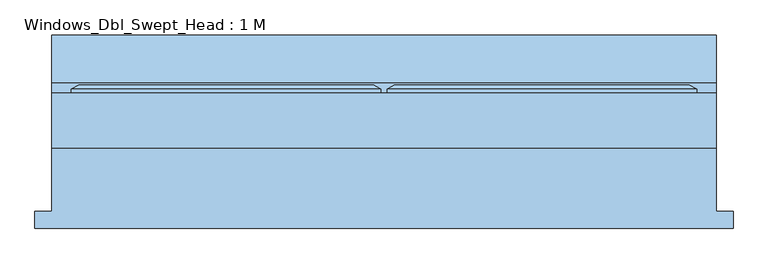
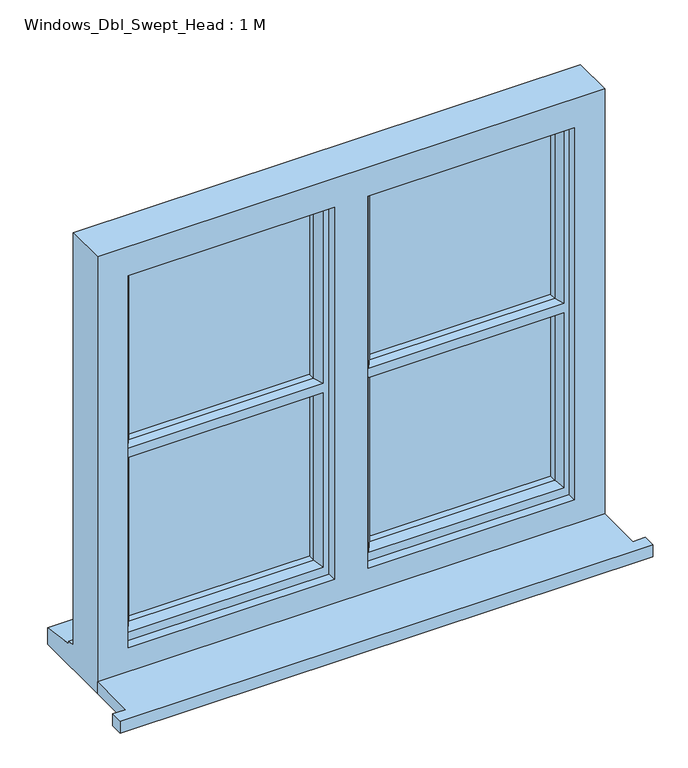
"""IFC4 building model written with IfcOpenShell, lengths in millimetres: window geometry, Windows_Dbl_Swept_Head : 1 M."""

from ifc_helpers import new_model, si_unit, frame, origin, place, context, project, spatial, polyline, circle_curve, outline, extrude, faceted_brep, source, transform, mapped, element, save
from ifc_brep_helpers import plane_surface, revolved_surface, advanced_brep


def windows_dbl_swept_head_1_m_37dff1ae(model_context):
    return source(origin(), model_context, "Body", "SolidModel", [
        extrude(outline(polyline([(-810.0, -130.8434322), (-810.0, -105.8434322), (-785.0, -105.8434322), (-785.0, -10.2434322), (215.0, -10.2434322), (215.0, -105.8434322), (240.0, -105.8434322), (240.0, -130.8434322), (-810.0, -130.8434322)])), frame((0.0, 0.0, 1200.0), z_axis=(0.0, 0.0, 1.0), x_axis=(1.0, 0.0, 0.0)), (0.0, 0.0, 1.0), 25.0),
        extrude(outline(polyline([(145.1480377, 36.7565678), (-240.0, 36.7565678), (-240.0, 60.7565678), (145.1480377, 60.7565678), (145.1480377, 36.7565678)])), frame((0.0, 0.0, 1293.0), z_axis=(0.0, 0.0, 1.0), x_axis=(1.0, 0.0, 0.0)), (0.0, 0.0, 1.0), 365.5),
        extrude(outline(polyline([(145.1480377, 36.7565678), (-240.0, 36.7565678), (-240.0, 60.7565678), (145.1480377, 60.7565678), (145.1480377, 36.7565678)])), frame((0.0, 0.0, 1674.5), z_axis=(0.0, 0.0, 1.0), x_axis=(1.0, 0.0, 0.0)), (0.0, 0.0, 1.0), 365.5),
        extrude(outline(polyline([(-330.0, 36.7565678), (-715.0, 36.7565678), (-715.0, 60.7565678), (-330.0, 60.7565678), (-330.0, 36.7565678)])), frame((0.0, 0.0, 1674.5), z_axis=(0.0, 0.0, 1.0), x_axis=(1.0, 0.0, 0.0)), (0.0, 0.0, 1.0), 365.5),
        extrude(outline(polyline([(-330.0, 36.7565678), (-715.1480377, 36.7565678), (-715.1480377, 60.7565678), (-330.0, 60.7565678), (-330.0, 36.7565678)])), frame((0.0, 0.0, 1292.8519623), z_axis=(0.0, 0.0, 1.0), x_axis=(1.0, 0.0, 0.0)), (0.0, 0.0, 1.0), 365.6480377),
        faceted_brep([(-785.0, -10.2434322, 1200.0), (215.0, -10.2434322, 1200.0), (215.0, -10.2434322, 2110.0), (-785.0, -10.2434322, 2110.0), (-318.0, -10.2434322, 2050.0), (-318.0, -10.2434322, 1275.0), (-725.0, -10.2434322, 1275.0), (-725.0, -10.2434322, 2050.0), (-252.0, -10.2434322, 2050.0), (155.0, -10.2434322, 2050.0), (155.0, -10.2434322, 1275.0), (-252.0, -10.2434322, 1275.0), (-785.0, 72.7565678, 2110.0), (-785.0, 72.7565678, 1251.0), (-785.0, 87.7565678, 1249.68767), (-785.0, 87.7565678, 1244.7449676), (-785.0, 160.2565678, 1233.8088847), (-785.0, 160.2565678, 1200.0), (215.0, 72.7565678, 2110.0), (215.0, 72.7565678, 1251.0), (-745.0, 72.7565678, 2070.0), (-745.0, 72.7565678, 1263.0), (-300.0, 72.7565678, 1263.0), (-300.0, 72.7565678, 2070.0), (-270.0, 72.7565678, 2070.0), (-270.0, 72.7565678, 1263.0), (175.0, 72.7565678, 1263.0), (175.0, 72.7565678, 2070.0), (-745.0, 7.7565678, 2070.0), (-745.0, 7.7565678, 1263.0), (-300.0, 7.7565678, 2070.0), (-300.0, 7.7565678, 1263.0), (-318.0, 7.7565678, 2050.0), (-725.0, 7.7565678, 2050.0), (-725.0, 7.7565678, 1275.0), (-318.0, 7.7565678, 1275.0), (-270.0, 7.7565678, 2070.0), (175.0, 7.7565678, 2070.0), (175.0, 7.7565678, 1263.0), (-270.0, 7.7565678, 1263.0), (155.0, 7.7565678, 2050.0), (-252.0, 7.7565678, 2050.0), (-252.0, 7.7565678, 1275.0), (155.0, 7.7565678, 1275.0), (215.0, 160.2565678, 1200.0), (215.0, 160.2565678, 1233.8088847), (215.0, 87.7565678, 1244.7449676), (215.0, 87.7565678, 1249.68767)], [[[0, 1, 2, 3], [4, 5, 6, 7], [8, 9, 10, 11]], [[0, 3, 12, 13, 14, 15, 16, 17]], [[13, 12, 18, 19], [20, 21, 22, 23], [24, 25, 26, 27]], [[21, 20, 28, 29]], [[28, 30, 31, 29], [32, 33, 34, 35]], [[36, 37, 38, 39], [40, 41, 42, 43]], [[33, 7, 6, 34]], [[12, 3, 2, 18]], [[28, 20, 23, 30]], [[27, 37, 36, 24]], [[7, 33, 32, 4]], [[40, 9, 8, 41]], [[19, 18, 2, 1, 44, 45, 46, 47]], [[27, 26, 38, 37]], [[9, 40, 43, 10]], [[23, 22, 31, 30]], [[25, 24, 36, 39]], [[41, 8, 11, 42]], [[4, 32, 35, 5]], [[44, 1, 0, 17]], [[45, 44, 17, 16]], [[46, 45, 16, 15]], [[47, 46, 15, 14]], [[19, 47, 14, 13]], [[22, 21, 29, 31]], [[26, 25, 39, 38]], [[11, 10, 43, 42]], [[35, 34, 6, 5]]]),
        advanced_brep(
        [(-280.0, 72.7565678, 2080.0), (-280.0, 78.5300705, 2080.0), (-280.0, 78.5300705, 1253.0), (-280.0, 72.7565678, 1253.0), (-270.0, 7.7565678, 2070.0), (-270.0, 72.7565678, 2070.0), (-270.0, 72.7565678, 1263.0), (-270.0, 7.7565678, 1263.0), (-230.0, 22.2494677, 2030.0), (-240.1480377, 7.7565678, 2040.1480377), (-240.1480377, 7.7565678, 1676.3519623), (-230.0, 22.2494677, 1681.5), (-240.1480377, 7.7565678, 1292.8519623), (-230.0, 22.2494677, 1303.0), (-230.0, 22.2494677, 1651.5), (-240.1480377, 7.7565678, 1656.6480377), (-230.0, 36.7565678, 2030.0), (-230.0, 36.7565678, 1681.5), (-230.0, 36.7565678, 1303.0), (-230.0, 36.7565678, 1651.5), (-240.0, 60.7565678, 2040.0), (-240.0, 36.7565678, 2040.0), (-240.0, 36.7565678, 1674.5), (-240.0, 60.7565678, 1674.5), (-240.0, 36.7565678, 1293.0), (-240.0, 60.7565678, 1293.0), (-240.0, 60.7565678, 1658.5), (-240.0, 36.7565678, 1658.5), (-230.0, 60.7565678, 1303.0), (-230.0, 78.5300705, 1303.0), (-230.0, 78.5300705, 1651.5), (-230.0, 60.7565678, 1651.5), (-230.0, 60.7565678, 1681.5), (-230.0, 78.5300705, 1681.5), (-230.0, 78.5300705, 2000.791203), (-230.0, 60.7565678, 2000.791203), (-247.4457548, 84.3035732, 2047.4457548), (-230.0, 78.5300705, 2030.0), (-235.0, 80.1847718, 1681.5), (-247.4457548, 84.3035732, 1669.0542452), (-247.4457548, 84.3035732, 1285.5542452), (-247.4457548, 84.3035732, 1663.9457548), (-235.0, 80.1847718, 1651.5), (-269.2153903, 84.3035732, 2069.2153903), (-269.2153903, 84.3035732, 1263.7846097), (185.0, 78.5300705, 1253.0), (185.0, 72.7565678, 1253.0), (175.0, 72.7565678, 1263.0), (175.0, 7.7565678, 1263.0), (145.1480377, 7.7565678, 1292.8519623), (135.0, 22.2494677, 1303.0), (135.0, 36.7565678, 1303.0), (145.0, 36.7565678, 1293.0), (145.0, 60.7565678, 1293.0), (135.0, 60.7565678, 1303.0), (135.0, 78.5300705, 1303.0), (152.4457548, 84.3035732, 1285.5542452), (174.2153903, 84.3035732, 1263.7846097), (185.0, 78.5300705, 2080.0), (185.0, 72.7565678, 2080.0), (175.0, 72.7565678, 2070.0), (175.0, 7.7565678, 2070.0), (145.1480377, 7.7565678, 1656.6480377), (135.0, 22.2494677, 1651.5), (145.1480377, 7.7565678, 2040.1480377), (135.0, 22.2494677, 2030.0), (135.0, 22.2494677, 1681.5), (145.1480377, 7.7565678, 1676.3519623), (135.0, 36.7565678, 1651.5), (135.0, 36.7565678, 2030.0), (135.0, 36.7565678, 1681.5), (145.0, 36.7565678, 1658.5), (145.0, 60.7565678, 1658.5), (145.0, 36.7565678, 2040.0), (145.0, 60.7565678, 2040.0), (145.0, 60.7565678, 1674.5), (145.0, 36.7565678, 1674.5), (135.0, 60.7565678, 1651.5), (135.0, 78.5300705, 1651.5), (135.0, 78.5300705, 1681.5), (135.0, 60.7565678, 1681.5), (135.0, 60.7565678, 2000.791203), (135.0, 78.5300705, 2000.791203), (140.0, 80.1847718, 1651.5), (152.4457548, 84.3035732, 1663.9457548), (135.0, 78.5300705, 2030.0), (152.4457548, 84.3035732, 2047.4457548), (152.4457548, 84.3035732, 1669.0542452), (140.0, 80.1847718, 1681.5), (174.2153903, 84.3035732, 2069.2153903)],
        [
            (0, 1),
            (1, 2),
            (2, 3),
            (3, 0),
            (4, 5),
            (5, 6),
            (6, 7),
            (7, 4),
            (8, 9),
            (9, 10),
            (10, 11),
            (11, 8),
            (12, 13),
            (13, 14),
            (14, 15),
            (15, 12),
            (16, 8),
            (11, 17),
            (17, 16),
            (13, 18),
            (18, 19),
            (19, 14),
            (20, 21),
            (21, 22),
            (22, 23),
            (23, 20),
            (24, 25),
            (25, 26),
            (26, 27),
            (27, 24),
            (28, 29),
            (29, 30),
            (30, 31),
            (31, 28),
            (32, 33),
            (33, 34),
            (34, 35),
            (35, 32),
            (36, 37),
            (37, 34),
            (33, 38),
            (38, 39),
            (39, 36),
            (29, 40),
            (40, 41),
            (41, 42),
            (42, 30),
            (1, 43),
            (43, 44),
            (44, 2),
            (2, 45),
            (45, 46),
            (46, 3),
            (6, 47),
            (47, 48),
            (48, 7),
            (12, 49),
            (49, 50),
            (50, 13),
            (50, 51),
            (51, 18),
            (24, 52),
            (52, 53),
            (53, 25),
            (28, 54),
            (54, 55),
            (55, 29),
            (55, 56),
            (56, 40),
            (44, 57),
            (57, 45),
            (45, 58),
            (58, 59),
            (59, 46),
            (47, 60),
            (60, 61),
            (61, 48),
            (49, 62),
            (62, 63),
            (63, 50),
            (64, 65),
            (65, 66),
            (66, 67),
            (67, 64),
            (63, 68),
            (68, 51),
            (65, 69),
            (69, 70),
            (70, 66),
            (52, 71),
            (71, 72),
            (72, 53),
            (73, 74),
            (74, 75),
            (75, 76),
            (76, 73),
            (54, 77),
            (77, 78),
            (78, 55),
            (79, 80),
            (80, 81),
            (81, 82),
            (82, 79),
            (78, 83),
            (83, 84),
            (84, 56),
            (85, 86),
            (86, 87),
            (87, 88),
            (88, 79),
            (82, 85),
            (57, 89),
            (89, 58),
            (0, 59),
            (58, 1),
            (5, 60),
            (4, 61),
            (15, 62),
            (9, 64),
            (67, 10),
            (8, 65),
            (16, 69),
            (27, 71),
            (68, 19),
            (21, 73),
            (76, 22),
            (17, 70),
            (20, 74),
            (72, 26),
            (31, 77),
            (23, 75),
            (80, 32),
            (35, 81, circle_curve(frame((-47.5, 60.7565678, 1325.0), z_axis=(0.0, 1.0, 0.0), x_axis=(1.0, 0.0, 0.0)), 700.0)),
            (36, 86),
            (85, 37),
            (43, 89),
            (84, 41),
            (39, 87),
            (38, 88),
            (11, 66),
            (14, 63),
            (42, 83),
            (82, 34, circle_curve(frame((-47.5, 78.5300705, 1325.0), z_axis=(0.0, -1.0, 0.0), x_axis=(1.0, 0.0, 0.0)), 700.0)),
        ],
        [
            plane_surface(frame((-280.0, 78.5300705, 2080.0), z_axis=(-1.0, 0.0, 0.0), x_axis=(0.0, 0.0, -1.0))),
            plane_surface(frame((-270.0, 72.7565678, 2070.0), z_axis=(-1.0, 0.0, 0.0), x_axis=(0.0, 0.0, -1.0))),
            plane_surface(frame((-240.1480377, 7.7565678, 2040.1480377), z_axis=(0.8191520442889492, -0.5735764363511071, 0.0), x_axis=(0.0, 0.0, -1.0))),
            plane_surface(frame((-230.0, 22.2494677, 2030.0), z_axis=(1.0, 0.0, 0.0), x_axis=(0.0, 0.0, -1.0))),
            plane_surface(frame((-240.0, 36.7565678, 2040.0), z_axis=(1.0, 0.0, 0.0), x_axis=(0.0, 0.0, -1.0))),
            plane_surface(frame((-230.0, 60.7565678, 2030.0), z_axis=(1.0, 0.0, 0.0), x_axis=(0.0, 0.0, -1.0))),
            plane_surface(frame((-230.0, 78.5300705, 2030.0), z_axis=(0.31418232948755237, 0.9493626619147053, 0.0), x_axis=(0.0, 0.0, -1.0))),
            plane_surface(frame((-269.2153903, 84.3035732, 2069.2153903), z_axis=(-0.47196942945730275, 0.8816149146071363, 0.0), x_axis=(0.0, 0.0, -1.0))),
            plane_surface(frame((-280.0, 78.5300705, 1253.0), z_axis=(0.0, 0.0, -1.0), x_axis=(1.0, 0.0, 0.0))),
            plane_surface(frame((-270.0, 72.7565678, 1263.0), z_axis=(0.0, 0.0, -1.0), x_axis=(1.0, 0.0, 0.0))),
            plane_surface(frame((-240.1480377, 7.7565678, 1292.8519623), z_axis=(0.0, -0.5735764363511044, 0.819152044288951), x_axis=(1.0, 0.0, 0.0))),
            plane_surface(frame((-230.0, 22.2494677, 1303.0), z_axis=(0.0, 0.0, 1.0), x_axis=(1.0, 0.0, 0.0))),
            plane_surface(frame((-240.0, 36.7565678, 1293.0), z_axis=(0.0, 0.0, 1.0), x_axis=(1.0, 0.0, 0.0))),
            plane_surface(frame((-230.0, 60.7565678, 1303.0), z_axis=(0.0, 0.0, 1.0), x_axis=(1.0, 0.0, 0.0))),
            plane_surface(frame((-230.0, 78.5300705, 1303.0), z_axis=(0.0, 0.9493626619147063, 0.31418232948754926), x_axis=(1.0, 0.0, 0.0))),
            plane_surface(frame((-269.2153903, 84.3035732, 1263.7846097), z_axis=(0.0, 0.8816149146071347, -0.47196942945730563), x_axis=(1.0, 0.0, 0.0))),
            plane_surface(frame((185.0, 78.5300705, 1253.0), z_axis=(1.0, 0.0, 0.0), x_axis=(0.0, 0.0, 1.0))),
            plane_surface(frame((175.0, 72.7565678, 1263.0), z_axis=(1.0, 0.0, 0.0), x_axis=(0.0, 0.0, 1.0))),
            plane_surface(frame((145.1480377, 7.7565678, 1292.8519623), z_axis=(-0.8191520442889529, -0.5735764363511018, 0.0), x_axis=(0.0, 0.0, 1.0))),
            plane_surface(frame((135.0, 22.2494677, 1303.0), z_axis=(-1.0, 0.0, 0.0), x_axis=(0.0, 0.0, 1.0))),
            plane_surface(frame((145.0, 36.7565678, 1293.0), z_axis=(-1.0, 0.0, 0.0), x_axis=(0.0, 0.0, 1.0))),
            plane_surface(frame((135.0, 60.7565678, 1303.0), z_axis=(-1.0, 0.0, 0.0), x_axis=(0.0, 0.0, 1.0))),
            plane_surface(frame((135.0, 78.5300705, 1303.0), z_axis=(-0.3141823294875462, 0.9493626619147074, 0.0), x_axis=(0.0, 0.0, 1.0))),
            plane_surface(frame((174.2153903, 84.3035732, 1263.7846097), z_axis=(0.4719694294573085, 0.8816149146071331, 0.0), x_axis=(0.0, 0.0, 1.0))),
            plane_surface(frame((185.0, 78.5300705, 2080.0), z_axis=(0.0, 0.0, 1.0), x_axis=(-1.0, 0.0, 0.0))),
            plane_surface(frame((185.0, 72.7565678, 2080.0), z_axis=(0.0, -1.0, 0.0), x_axis=(-1.0, 0.0, 0.0))),
            plane_surface(frame((175.0, 72.7565678, 2070.0), z_axis=(0.0, 0.0, 1.0), x_axis=(-1.0, 0.0, 0.0))),
            plane_surface(frame((175.0, 7.7565678, 2070.0), z_axis=(0.0, -1.0, 0.0), x_axis=(-1.0, 0.0, 0.0))),
            plane_surface(frame((145.1480377, 7.7565678, 2040.1480377), z_axis=(0.0, -0.5735764363511044, -0.819152044288951), x_axis=(-1.0, 0.0, 0.0))),
            plane_surface(frame((135.0, 22.2494677, 2030.0), z_axis=(0.0, 0.0, -1.0), x_axis=(-1.0, 0.0, 0.0))),
            plane_surface(frame((135.0, 36.7565678, 2030.0), z_axis=(0.0, 1.0, 0.0), x_axis=(-1.0, 0.0, 0.0))),
            plane_surface(frame((145.0, 36.7565678, 2040.0), z_axis=(0.0, 0.0, -1.0), x_axis=(-1.0, 0.0, 0.0))),
            plane_surface(frame((145.0, 60.7565678, 2040.0), z_axis=(0.0, -1.0, 0.0), x_axis=(-1.0, 0.0, 0.0))),
            plane_surface(frame((135.0, 78.5300705, 2030.0), z_axis=(0.0, 0.9493626619147064, -0.3141823294875493), x_axis=(-1.0, 0.0, 0.0))),
            plane_surface(frame((152.4457548, 84.3035732, 2047.4457548), z_axis=(0.0, 1.0, 0.0), x_axis=(-1.0, 0.0, 0.0))),
            plane_surface(frame((174.2153903, 84.3035732, 2069.2153903), z_axis=(0.0, 0.8816149146071347, 0.47196942945730563), x_axis=(-1.0, 0.0, 0.0))),
            plane_surface(frame((152.4457548, 84.3035732, 1669.0542452), z_axis=(0.0, 0.9493626619145938, 0.3141823294878896), x_axis=(-1.0, 0.0, 0.0))),
            plane_surface(frame((152.4457548, 80.1847718, 1681.5), z_axis=(0.0, 0.0, 1.0), x_axis=(-1.0, 0.0, 0.0))),
            plane_surface(frame((152.4457548, 60.7565678, 1674.5), z_axis=(0.0, 0.0, 1.0), x_axis=(-1.0, 0.0, 0.0))),
            plane_surface(frame((152.4457548, 36.7565678, 1681.5), z_axis=(0.0, 0.0, 1.0), x_axis=(-1.0, 0.0, 0.0))),
            plane_surface(frame((152.4457548, 22.2494677, 1681.5), z_axis=(0.0, -0.33472142672711697, 0.9423171262848634), x_axis=(-1.0, 0.0, 0.0))),
            plane_surface(frame((152.4457548, 7.7565678, 1656.6480377), z_axis=(0.0, -0.33472142672499106, -0.9423171262856186), x_axis=(-1.0, 0.0, 0.0))),
            plane_surface(frame((152.4457548, 22.2494677, 1651.5), z_axis=(0.0, 0.0, -1.0), x_axis=(-1.0, 0.0, 0.0))),
            plane_surface(frame((152.4457548, 36.7565678, 1658.5), z_axis=(0.0, 0.0, -1.0), x_axis=(-1.0, 0.0, 0.0))),
            plane_surface(frame((152.4457548, 60.7565678, 1651.5), z_axis=(0.0, 0.0, -1.0), x_axis=(-1.0, 0.0, 0.0))),
            plane_surface(frame((152.4457548, 80.1847718, 1651.5), z_axis=(0.0, 0.9493626619148547, -0.31418232948710106), x_axis=(-1.0, 0.0, 0.0))),
            plane_surface(frame((-230.0, 78.5300705, 2030.0), z_axis=(0.0, 1.0, 0.0), x_axis=(0.0, 0.0, 1.0))),
            revolved_surface(polyline([(652.5, 78.5300705, 1325.0), (652.5, 60.7565678, 1325.0)]), (-47.5, 78.5300705, 1325.0), (0.0, 1.0, 0.0)),
        ],
        [
            (0, [[1, 2, 3, 4]]),
            (1, [[5, 6, 7, 8]]),
            (2, [[9, 10, 11, 12]]),
            (2, [[13, 14, 15, 16]]),
            (3, [[17, -12, 18, 19]]),
            (3, [[20, 21, 22, -14]]),
            (4, [[23, 24, 25, 26]]),
            (4, [[27, 28, 29, 30]]),
            (5, [[31, 32, 33, 34]]),
            (5, [[35, 36, 37, 38]]),
            (6, [[39, 40, -36, 41, 42, 43]]),
            (6, [[44, 45, 46, 47, -32]]),
            (7, [[-2, 48, 49, 50]]),
            (8, [[-3, 51, 52, 53]]),
            (9, [[-7, 54, 55, 56]]),
            (10, [[-13, 57, 58, 59]]),
            (11, [[-20, -59, 60, 61]]),
            (12, [[-27, 62, 63, 64]]),
            (13, [[-31, 65, 66, 67]]),
            (14, [[-44, -67, 68, 69]]),
            (15, [[-50, 70, 71, -51]]),
            (16, [[-52, 72, 73, 74]]),
            (17, [[-55, 75, 76, 77]]),
            (18, [[-58, 78, 79, 80]]),
            (18, [[81, 82, 83, 84]]),
            (19, [[-60, -80, 85, 86]]),
            (19, [[87, 88, 89, -82]]),
            (20, [[-63, 90, 91, 92]]),
            (20, [[93, 94, 95, 96]]),
            (21, [[-66, 97, 98, 99]]),
            (21, [[100, 101, 102, 103]]),
            (22, [[-68, -99, 104, 105, 106]]),
            (22, [[107, 108, 109, 110, -103, 111]]),
            (23, [[-71, 112, 113, -72]]),
            (24, [[-1, 114, -73, 115]]),
            (25, [[-4, -53, -74, -114], [-6, 116, -75, -54]]),
            (26, [[-5, 117, -76, -116]]),
            (27, [[-8, -56, -77, -117], [-57, -16, 118, -78], [119, -84, 120, -10]]),
            (28, [[-9, 121, -81, -119]]),
            (29, [[-17, 122, -87, -121]]),
            (30, [[-62, -30, 123, -90], [-61, -86, 124, -21]]),
            (30, [[125, -96, 126, -24], [-122, -19, 127, -88]]),
            (31, [[-23, 128, -93, -125]]),
            (32, [[-64, -92, 129, -28], [-65, -34, 130, -97]]),
            (32, [[-128, -26, 131, -94], [132, -38, 133, -101]]),
            (33, [[-39, 134, -107, 135]]),
            (34, [[-49, 136, -112, -70], [-69, -106, 137, -45], [-134, -43, 138, -108]]),
            (35, [[-48, -115, -113, -136]]),
            (36, [[-138, -42, 139, -109]]),
            (37, [[-132, -100, -110, -139, -41, -35]]),
            (38, [[-25, -126, -95, -131]]),
            (39, [[140, -89, -127, -18]]),
            (40, [[-120, -83, -140, -11]]),
            (41, [[-118, -15, 141, -79]]),
            (42, [[-141, -22, -124, -85]]),
            (43, [[-29, -129, -91, -123]]),
            (44, [[-130, -33, -47, 142, -104, -98]]),
            (45, [[-137, -105, -142, -46]]),
            (46, [[143, -40, -135, -111]]),
            (47, [[-133, -37, -143, -102]]),
        ],
    ),
        advanced_brep(
        [(-330.0, 60.7565678, 2040.0), (-715.0, 60.7565678, 2040.0), (-715.0, 60.7565678, 1674.5), (-330.0, 60.7565678, 1674.5), (-705.0, 60.7565678, 2000.791203), (-340.0, 60.7565678, 2000.791203), (-340.0, 60.7565678, 1681.5), (-705.0, 60.7565678, 1681.5), (-715.0, 60.7565678, 1293.0), (-330.0, 60.7565678, 1293.0), (-330.0, 60.7565678, 1658.5), (-715.0, 60.7565678, 1658.5), (-340.0, 60.7565678, 1303.0), (-705.0, 60.7565678, 1303.0), (-705.0, 60.7565678, 1651.5), (-340.0, 60.7565678, 1651.5), (-755.0, 72.7565678, 2080.0), (-755.0, 78.5300705, 2080.0), (-755.0, 78.5300705, 1253.0), (-755.0, 72.7565678, 1253.0), (-745.0, 7.7565678, 2070.0), (-745.0, 72.7565678, 2070.0), (-745.0, 72.7565678, 1263.0), (-745.0, 7.7565678, 1263.0), (-705.0, 22.2494677, 2030.0), (-715.1480377, 7.7565678, 2040.1480377), (-715.1480377, 7.7565678, 1676.3519623), (-705.0, 22.2494677, 1681.5), (-715.1480377, 7.7565678, 1292.8519623), (-705.0, 22.2494677, 1303.0), (-705.0, 22.2494677, 1651.5), (-715.1480377, 7.7565678, 1656.6480377), (-705.0, 36.7565678, 2030.0), (-705.0, 36.7565678, 1681.5), (-705.0, 36.7565678, 1303.0), (-705.0, 36.7565678, 1651.5), (-715.0, 36.7565678, 2040.0), (-715.0, 36.7565678, 1674.5), (-715.0, 36.7565678, 1293.0), (-715.0, 36.7565678, 1658.5), (-705.0, 78.5300705, 1303.0), (-705.0, 78.5300705, 1651.5), (-705.0, 78.5300705, 1681.5), (-705.0, 78.5300705, 2000.791203), (-722.4457548, 84.3035732, 2047.4457548), (-705.0, 78.5300705, 2030.0), (-710.0, 80.1847718, 1681.5), (-722.4457548, 84.3035732, 1669.0542452), (-722.4457548, 84.3035732, 1285.5542452), (-722.4457548, 84.3035732, 1663.9457548), (-710.0, 80.1847718, 1651.5), (-744.2153903, 84.3035732, 2069.2153903), (-744.2153903, 84.3035732, 1263.7846097), (-290.0, 78.5300705, 1253.0), (-290.0, 72.7565678, 1253.0), (-300.0, 72.7565678, 1263.0), (-300.0, 7.7565678, 1263.0), (-329.8519623, 7.7565678, 1292.8519623), (-340.0, 22.2494677, 1303.0), (-340.0, 36.7565678, 1303.0), (-330.0, 36.7565678, 1293.0), (-340.0, 78.5300705, 1303.0), (-322.5542452, 84.3035732, 1285.5542452), (-300.7846097, 84.3035732, 1263.7846097), (-290.0, 78.5300705, 2080.0), (-290.0, 72.7565678, 2080.0), (-300.0, 72.7565678, 2070.0), (-300.0, 7.7565678, 2070.0), (-329.8519623, 7.7565678, 1656.6480377), (-340.0, 22.2494677, 1651.5), (-329.8519623, 7.7565678, 2040.1480377), (-340.0, 22.2494677, 2030.0), (-340.0, 22.2494677, 1681.5), (-329.8519623, 7.7565678, 1676.3519623), (-340.0, 36.7565678, 1651.5), (-340.0, 36.7565678, 2030.0), (-340.0, 36.7565678, 1681.5), (-330.0, 36.7565678, 1658.5), (-330.0, 36.7565678, 2040.0), (-330.0, 36.7565678, 1674.5), (-340.0, 78.5300705, 1651.5), (-340.0, 78.5300705, 1681.5), (-340.0, 78.5300705, 2000.791203), (-335.0, 80.1847718, 1651.5), (-322.5542452, 84.3035732, 1663.9457548), (-340.0, 78.5300705, 2030.0), (-322.5542452, 84.3035732, 2047.4457548), (-322.5542452, 84.3035732, 1669.0542452), (-335.0, 80.1847718, 1681.5), (-300.7846097, 84.3035732, 2069.2153903)],
        [
            (0, 1),
            (1, 2),
            (2, 3),
            (3, 0),
            (4, 5, circle_curve(frame((-522.5, 60.7565678, 1325.0), z_axis=(0.0, 1.0, 0.0), x_axis=(1.0, 0.0, 0.0)), 700.0)),
            (5, 6),
            (6, 7),
            (7, 4),
            (8, 9),
            (9, 10),
            (10, 11),
            (11, 8),
            (12, 13),
            (13, 14),
            (14, 15),
            (15, 12),
            (16, 17),
            (17, 18),
            (18, 19),
            (19, 16),
            (20, 21),
            (21, 22),
            (22, 23),
            (23, 20),
            (24, 25),
            (25, 26),
            (26, 27),
            (27, 24),
            (28, 29),
            (29, 30),
            (30, 31),
            (31, 28),
            (32, 24),
            (27, 33),
            (33, 32),
            (29, 34),
            (34, 35),
            (35, 30),
            (1, 36),
            (36, 37),
            (37, 2),
            (38, 8),
            (11, 39),
            (39, 38),
            (13, 40),
            (40, 41),
            (41, 14),
            (7, 42),
            (42, 43),
            (43, 4),
            (44, 45),
            (45, 43),
            (42, 46),
            (46, 47),
            (47, 44),
            (40, 48),
            (48, 49),
            (49, 50),
            (50, 41),
            (17, 51),
            (51, 52),
            (52, 18),
            (18, 53),
            (53, 54),
            (54, 19),
            (22, 55),
            (55, 56),
            (56, 23),
            (28, 57),
            (57, 58),
            (58, 29),
            (58, 59),
            (59, 34),
            (38, 60),
            (60, 9),
            (12, 61),
            (61, 40),
            (61, 62),
            (62, 48),
            (52, 63),
            (63, 53),
            (53, 64),
            (64, 65),
            (65, 54),
            (55, 66),
            (66, 67),
            (67, 56),
            (57, 68),
            (68, 69),
            (69, 58),
            (70, 71),
            (71, 72),
            (72, 73),
            (73, 70),
            (69, 74),
            (74, 59),
            (71, 75),
            (75, 76),
            (76, 72),
            (60, 77),
            (77, 10),
            (78, 0),
            (3, 79),
            (79, 78),
            (15, 80),
            (80, 61),
            (81, 6),
            (5, 82),
            (82, 81),
            (80, 83),
            (83, 84),
            (84, 62),
            (85, 86),
            (86, 87),
            (87, 88),
            (88, 81),
            (82, 85),
            (63, 89),
            (89, 64),
            (16, 65),
            (64, 17),
            (21, 66),
            (20, 67),
            (31, 68),
            (25, 70),
            (73, 26),
            (24, 71),
            (32, 75),
            (39, 77),
            (74, 35),
            (36, 78),
            (79, 37),
            (33, 76),
            (44, 86),
            (85, 45),
            (51, 89),
            (84, 49),
            (47, 87),
            (46, 88),
            (83, 50),
            (69, 30),
            (72, 27),
            (82, 43, circle_curve(frame((-522.5, 78.5300705, 1325.0), z_axis=(0.0, -1.0, 0.0), x_axis=(1.0, 0.0, 0.0)), 700.0)),
        ],
        [
            plane_surface(frame((145.0, 60.7565678, 2040.0), z_axis=(0.0, -1.0, 0.0), x_axis=(-1.0, 0.0, 0.0))),
            plane_surface(frame((-755.0, 78.5300705, 2080.0), z_axis=(-1.0, 0.0, 0.0), x_axis=(0.0, 0.0, -1.0))),
            plane_surface(frame((-745.0, 72.7565678, 2070.0), z_axis=(-1.0, 0.0, 0.0), x_axis=(0.0, 0.0, -1.0))),
            plane_surface(frame((-715.1480377, 7.7565678, 2040.1480377), z_axis=(0.8191520442889492, -0.5735764363511071, 0.0), x_axis=(0.0, 0.0, -1.0))),
            plane_surface(frame((-705.0, 22.2494677, 2030.0), z_axis=(1.0, 0.0, 0.0), x_axis=(0.0, 0.0, -1.0))),
            plane_surface(frame((-715.0, 36.7565678, 2040.0), z_axis=(1.0, 0.0, 0.0), x_axis=(0.0, 0.0, -1.0))),
            plane_surface(frame((-705.0, 60.7565678, 2030.0), z_axis=(1.0, 0.0, 0.0), x_axis=(0.0, 0.0, -1.0))),
            plane_surface(frame((-705.0, 78.5300705, 2030.0), z_axis=(0.31418232948755237, 0.9493626619147053, 0.0), x_axis=(0.0, 0.0, -1.0))),
            plane_surface(frame((-744.2153903, 84.3035732, 2069.2153903), z_axis=(-0.47196942945730275, 0.8816149146071363, 0.0), x_axis=(0.0, 0.0, -1.0))),
            plane_surface(frame((-755.0, 78.5300705, 1253.0), z_axis=(0.0, 0.0, -1.0), x_axis=(1.0, 0.0, 0.0))),
            plane_surface(frame((-745.0, 72.7565678, 1263.0), z_axis=(0.0, 0.0, -1.0), x_axis=(1.0, 0.0, 0.0))),
            plane_surface(frame((-715.1480377, 7.7565678, 1292.8519623), z_axis=(0.0, -0.5735764363511044, 0.819152044288951), x_axis=(1.0, 0.0, 0.0))),
            plane_surface(frame((-705.0, 22.2494677, 1303.0), z_axis=(0.0, 0.0, 1.0), x_axis=(1.0, 0.0, 0.0))),
            plane_surface(frame((-715.0, 36.7565678, 1293.0), z_axis=(0.0, 0.0, 1.0), x_axis=(1.0, 0.0, 0.0))),
            plane_surface(frame((-705.0, 60.7565678, 1303.0), z_axis=(0.0, 0.0, 1.0), x_axis=(1.0, 0.0, 0.0))),
            plane_surface(frame((-705.0, 78.5300705, 1303.0), z_axis=(0.0, 0.9493626619147063, 0.31418232948754926), x_axis=(1.0, 0.0, 0.0))),
            plane_surface(frame((-744.2153903, 84.3035732, 1263.7846097), z_axis=(0.0, 0.8816149146071347, -0.47196942945730563), x_axis=(1.0, 0.0, 0.0))),
            plane_surface(frame((-290.0, 78.5300705, 1253.0), z_axis=(1.0, 0.0, 0.0), x_axis=(0.0, 0.0, 1.0))),
            plane_surface(frame((-300.0, 72.7565678, 1263.0), z_axis=(1.0, 0.0, 0.0), x_axis=(0.0, 0.0, 1.0))),
            plane_surface(frame((-329.8519623, 7.7565678, 1292.8519623), z_axis=(-0.8191520442889529, -0.5735764363511018, 0.0), x_axis=(0.0, 0.0, 1.0))),
            plane_surface(frame((-340.0, 22.2494677, 1303.0), z_axis=(-1.0, 0.0, 0.0), x_axis=(0.0, 0.0, 1.0))),
            plane_surface(frame((-330.0, 36.7565678, 1293.0), z_axis=(-1.0, 0.0, 0.0), x_axis=(0.0, 0.0, 1.0))),
            plane_surface(frame((-340.0, 60.7565678, 1303.0), z_axis=(-1.0, 0.0, 0.0), x_axis=(0.0, 0.0, 1.0))),
            plane_surface(frame((-340.0, 78.5300705, 1303.0), z_axis=(-0.3141823294875462, 0.9493626619147074, 0.0), x_axis=(0.0, 0.0, 1.0))),
            plane_surface(frame((-300.7846097, 84.3035732, 1263.7846097), z_axis=(0.4719694294573085, 0.8816149146071331, 0.0), x_axis=(0.0, 0.0, 1.0))),
            plane_surface(frame((-290.0, 78.5300705, 2080.0), z_axis=(0.0, 0.0, 1.0), x_axis=(-1.0, 0.0, 0.0))),
            plane_surface(frame((-290.0, 72.7565678, 2080.0), z_axis=(0.0, -1.0, 0.0), x_axis=(-1.0, 0.0, 0.0))),
            plane_surface(frame((-300.0, 72.7565678, 2070.0), z_axis=(0.0, 0.0, 1.0), x_axis=(-1.0, 0.0, 0.0))),
            plane_surface(frame((-300.0, 7.7565678, 2070.0), z_axis=(0.0, -1.0, 0.0), x_axis=(-1.0, 0.0, 0.0))),
            plane_surface(frame((-329.8519623, 7.7565678, 2040.1480377), z_axis=(0.0, -0.5735764363511044, -0.819152044288951), x_axis=(-1.0, 0.0, 0.0))),
            plane_surface(frame((-340.0, 22.2494677, 2030.0), z_axis=(0.0, 0.0, -1.0), x_axis=(-1.0, 0.0, 0.0))),
            plane_surface(frame((-340.0, 36.7565678, 2030.0), z_axis=(0.0, 1.0, 0.0), x_axis=(-1.0, 0.0, 0.0))),
            plane_surface(frame((-330.0, 36.7565678, 2040.0), z_axis=(0.0, 0.0, -1.0), x_axis=(-1.0, 0.0, 0.0))),
            plane_surface(frame((-340.0, 78.5300705, 2030.0), z_axis=(0.0, 0.9493626619147064, -0.3141823294875493), x_axis=(-1.0, 0.0, 0.0))),
            plane_surface(frame((-322.5542452, 84.3035732, 2047.4457548), z_axis=(0.0, 1.0, 0.0), x_axis=(-1.0, 0.0, 0.0))),
            plane_surface(frame((-300.7846097, 84.3035732, 2069.2153903), z_axis=(0.0, 0.8816149146071347, 0.47196942945730563), x_axis=(-1.0, 0.0, 0.0))),
            plane_surface(frame((-722.4457548, 80.1847718, 1681.5), z_axis=(0.0, 0.9493626619144715, 0.31418232948825914), x_axis=(1.0, 0.0, 0.0))),
            plane_surface(frame((-722.4457548, 84.3035732, 1663.9457548), z_axis=(0.0, 0.949362661914977, -0.3141823294867314), x_axis=(1.0, 0.0, 0.0))),
            plane_surface(frame((-722.4457548, 80.1847718, 1651.5), z_axis=(0.0, 0.0, -1.0), x_axis=(1.0, 0.0, 0.0))),
            plane_surface(frame((-722.4457548, 60.7565678, 1658.5), z_axis=(0.0, 0.0, -1.0), x_axis=(1.0, 0.0, 0.0))),
            plane_surface(frame((-722.4457548, 36.7565678, 1651.5), z_axis=(0.0, 0.0, -1.0), x_axis=(1.0, 0.0, 0.0))),
            plane_surface(frame((-722.4457548, 22.2494677, 1651.5), z_axis=(0.0, -0.3347214267259168, -0.9423171262852897), x_axis=(1.0, 0.0, 0.0))),
            plane_surface(frame((-722.4457548, 7.7565678, 1676.3519623), z_axis=(0.0, -0.33472142672616695, 0.9423171262852009), x_axis=(1.0, 0.0, 0.0))),
            plane_surface(frame((-722.4457548, 22.2494677, 1681.5), z_axis=(0.0, 0.0, 1.0), x_axis=(1.0, 0.0, 0.0))),
            plane_surface(frame((-722.4457548, 36.7565678, 1674.5), z_axis=(0.0, 0.0, 1.0), x_axis=(1.0, 0.0, 0.0))),
            plane_surface(frame((-722.4457548, 60.7565678, 1681.5), z_axis=(0.0, 0.0, 1.0), x_axis=(1.0, 0.0, 0.0))),
            plane_surface(frame((-230.0, 78.5300705, 2030.0), z_axis=(0.0, 1.0, 0.0), x_axis=(0.0, 0.0, 1.0))),
            revolved_surface(polyline([(177.5, 78.5300705, 1325.0), (177.5, 60.7565678, 1325.0)]), (-522.5, 72.7565678, 1325.0), (0.0, 1.0, 0.0)),
        ],
        [
            (0, [[1, 2, 3, 4], [5, 6, 7, 8]]),
            (0, [[9, 10, 11, 12], [13, 14, 15, 16]]),
            (1, [[17, 18, 19, 20]]),
            (2, [[21, 22, 23, 24]]),
            (3, [[25, 26, 27, 28]]),
            (3, [[29, 30, 31, 32]]),
            (4, [[33, -28, 34, 35]]),
            (4, [[36, 37, 38, -30]]),
            (5, [[39, 40, 41, -2]]),
            (5, [[42, -12, 43, 44]]),
            (6, [[45, 46, 47, -14]]),
            (6, [[48, 49, 50, -8]]),
            (7, [[51, 52, -49, 53, 54, 55]]),
            (7, [[56, 57, 58, 59, -46]]),
            (8, [[-18, 60, 61, 62]]),
            (9, [[-19, 63, 64, 65]]),
            (10, [[-23, 66, 67, 68]]),
            (11, [[-29, 69, 70, 71]]),
            (12, [[-36, -71, 72, 73]]),
            (13, [[-42, 74, 75, -9]]),
            (14, [[-45, -13, 76, 77]]),
            (15, [[-56, -77, 78, 79]]),
            (16, [[-62, 80, 81, -63]]),
            (17, [[-64, 82, 83, 84]]),
            (18, [[-67, 85, 86, 87]]),
            (19, [[-70, 88, 89, 90]]),
            (19, [[91, 92, 93, 94]]),
            (20, [[-72, -90, 95, 96]]),
            (20, [[97, 98, 99, -92]]),
            (21, [[-75, 100, 101, -10]]),
            (21, [[102, -4, 103, 104]]),
            (22, [[-76, -16, 105, 106]]),
            (22, [[107, -6, 108, 109]]),
            (23, [[-78, -106, 110, 111, 112]]),
            (23, [[113, 114, 115, 116, -109, 117]]),
            (24, [[-81, 118, 119, -82]]),
            (25, [[-17, 120, -83, 121]]),
            (26, [[-20, -65, -84, -120], [-22, 122, -85, -66]]),
            (27, [[-21, 123, -86, -122]]),
            (28, [[-24, -68, -87, -123], [-69, -32, 124, -88], [125, -94, 126, -26]]),
            (29, [[-25, 127, -91, -125]]),
            (30, [[-33, 128, -97, -127]]),
            (31, [[-74, -44, 129, -100], [-73, -96, 130, -37]]),
            (31, [[131, -104, 132, -40], [-128, -35, 133, -98]]),
            (32, [[-39, -1, -102, -131]]),
            (33, [[-51, 134, -113, 135]]),
            (34, [[-61, 136, -118, -80], [-79, -112, 137, -57], [-134, -55, 138, -114]]),
            (35, [[-60, -121, -119, -136]]),
            (36, [[-138, -54, 139, -115]]),
            (37, [[-137, -111, 140, -58]]),
            (38, [[-15, -47, -59, -140, -110, -105]]),
            (39, [[-43, -11, -101, -129]]),
            (40, [[141, -38, -130, -95]]),
            (41, [[-124, -31, -141, -89]]),
            (42, [[-126, -93, 142, -27]]),
            (43, [[-142, -99, -133, -34]]),
            (44, [[-41, -132, -103, -3]]),
            (45, [[-7, -107, -116, -139, -53, -48]]),
            (46, [[143, -52, -135, -117]]),
            (47, [[-5, -50, -143, -108]]),
        ],
    ),
    ])


if __name__ == "__main__":
    model = new_model("IFC4")
    model_context = context("Model", 3, world=origin())
    ifc_project = project(units=[si_unit("LENGTHUNIT", "METRE", prefix="MILLI")], contexts=[model_context])
    site = spatial("IfcSite", under=ifc_project)
    building = spatial("IfcBuilding", under=site)
    placement = place(None, origin())
    windows_dbl_swept_head_1_m_shape = windows_dbl_swept_head_1_m_37dff1ae(model_context)
    element("IfcWindow", 1, ObjectType="Windows_Dbl_Swept_Head : 1 M", at=placement, inside=building, context=model_context, shape_type="MappedRepresentation", body=[
        mapped(windows_dbl_swept_head_1_m_shape, transform((0.0, 0.0, 0.0), x_axis=(1.0, 0.0, 0.0), y_axis=(0.0, 1.0, 0.0), z_axis=(0.0, 0.0, 1.0))),
    ])
    save(model, "model.ifc")

# Revit data of these elements
# Type "Windows_Dbl_Swept_Head : 1 M"
#   Type Mark = "67"
#   Operation = "DoublePanelVertical"
#   Construction Type Id = "GSP4R"
#   Manufacturer = "Revit"
#   Keynote = "L10"
#   Analytic Construction = "1/8 in Pilkington single glazing"
#   Wrap Layers (Ext) from Ext = 0.1025 m
#   Wrap Layers (Int) from Ext = 0.1775 m
#   Window Board Projection = 0.025 m
#   Window Board Extension = 0.025 m
#   Visual Light Transmittance = 0.9
#   Solar Heat Gain Coefficient = 0.78
#   Rough Width = 1.0 m
#   Rough Height = 0.91 m
#   Radius - Swept Head = 0.7 m
#   Height = 0.91 m
#   Width = 1.0 m
#   Heat Transfer Coefficient (U) = 3.6886 W/(m²·K)
#   Glazing Thickness = 0.024 m
#   FrameOffset - External = 0.05 m
#   Frame Depth = 0.065 m
#   Default Head Height = 2.11 m
#   Cill Depth = 0.0875 m
#   Cavity Closer Width = 0.05 m
#   Cavity Closer Offset from Ext = 0.1025 m
#   Cavity Closer Depth = 0.085 m
#   Vis - Cavity Closers = yes
#   Define Thermal Properties by = 1
#   Material Trim = Window Frame
#   Material Glass = Glass
#   Material Frame = Window Frame
#   Wall Closure = (empty or 0)
# Element 1 (IfcWindow, "Windows_Dbl_Swept_Head : 1 M")
#   Materials on its faces: "Window Frame", "Glass"
# Materials
#   "Window Frame": colour RGB 249 249 249, transparency 0, Keynote = "L10", Cost = 0
#   "Glass": class "Glass", colour RGB 0 128 192, transparency 0.9, Description = "Soda Lime Glass", Cost = 0
